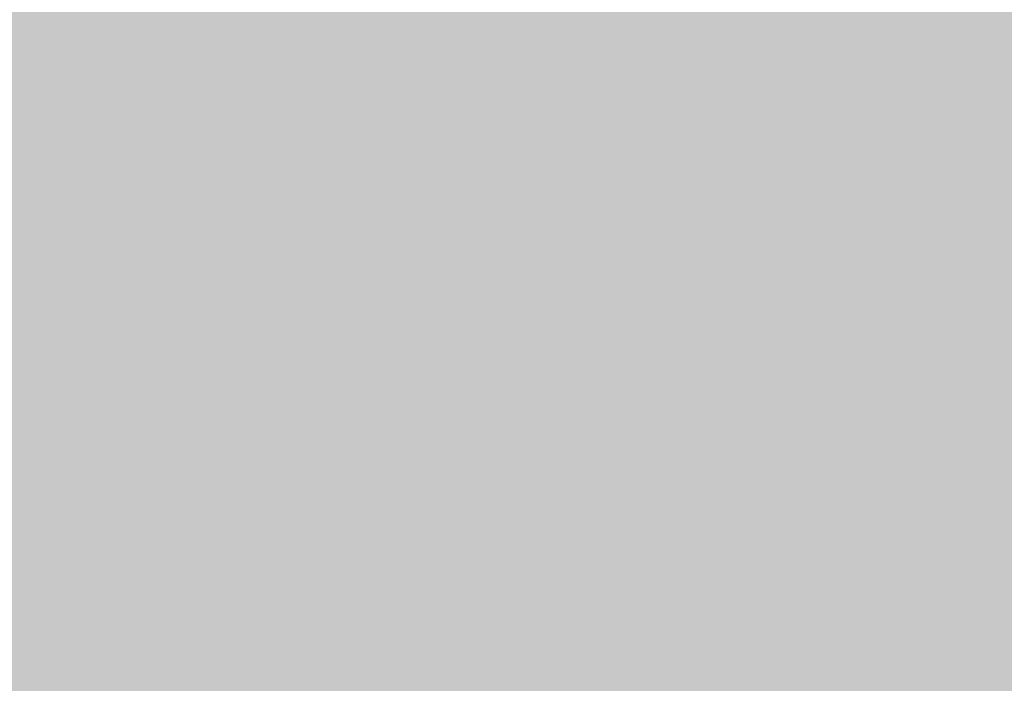
# Model space of a CAD drawing. Units: feet. Extents: x 3168 to 4724, y 827 to 1477.
# Tile 143 of 256: x 3301.1362 to 3301.138323, y 1099.01485 to 1099.016281. Entities that reach past the tile are written whole.
import ezdxf

# ---------------------------------------------------------------- set-up
doc = ezdxf.new("R2010")
doc.units = ezdxf.units.FT
doc.layers.add('A-ELEV', color=7, linetype='Continuous', lineweight=35)
doc.layers.add('A-ELEV-PATT', color=8, linetype='Continuous', lineweight=13)

msp = doc.modelspace()

# ---------------------------------------------------------------- hatches: boundary and pattern name
at = {"layer": 'A-ELEV-PATT'}
h = msp.add_hatch(color=256, dxfattribs=at)
h.dxf.hatch_style = 1
edge = h.paths.add_edge_path()
edge.add_ellipse((3552.9057615, 979.2201412), major_axis=(36.7449243, 0), ratio=0.4848484848, start_angle=0, end_angle=360)
edge = h.paths.add_edge_path()
edge.add_ellipse((3559.8916366, 929.2522824), major_axis=(36.7449243, 0), ratio=0.4848484848, start_angle=0, end_angle=360)
edge = h.paths.add_edge_path()
edge.add_line((3299.3168105, 1198.606081), (3479.9167135, 1198.606081))
edge.add_line((3479.9167135, 1198.606081), (3479.9167135, 1209.8685704))
edge.add_spline(control_points=[(3479.9167135, 1209.8685704), (3464.3011571, 1209.8685704), (3448.6856007, 1209.8685704), (3410.949139, 1209.8685704), (3388.8282339, 1209.8685704), (3355.6468761, 1209.8685704), (3344.5864235, 1209.8685704), (3327.9957446, 1209.8685704), (3322.4655183, 1209.8685704), (3314.1701788, 1209.8685704), (3311.4050657, 1209.8685704), (3307.257396, 1209.8685704), (3305.8748394, 1209.8685704), (3303.8010045, 1209.8685704), (3303.1097262, 1209.8685704), (3302.0728088, 1209.8685704), (3301.7271697, 1209.8685704), (3301.2087109, 1209.8685704), (3301.0358914, 1209.8685704), (3300.776662, 1209.8685704), (3300.6902522, 1209.8685704), (3300.5606376, 1209.8685704), (3300.5174327, 1209.8685704), (3300.4526253, 1209.8685704), (3300.4310229, 1209.8685704), (3300.3986192, 1209.8685704), (3300.387818, 1209.8685704), (3300.3662155, 1209.8685704), (3300.3456757, 1209.8685704), (3300.3455476, 1209.8685704), (3300.345505, 1209.8685704), (3300.3433041, 1209.8685704), (3300.341146, 1209.8685707), (3300.337909, 1209.8685714), (3300.33683, 1209.8685718), (3300.3339422, 1209.8685728), (3300.3321334, 1209.8685736), (3300.3255154, 1209.8685773), (3300.3207065, 1209.8685812), (3300.3109248, 1209.8685917), (3300.305952, 1209.8685984), (3300.2905113, 1209.8686233), (3300.2800452, 1209.8686461), (3300.2324255, 1209.868777), (3300.1952979, 1209.868954), (3299.9510684, 1209.8706077), (3299.7448244, 1209.8743259), (3299.4368271, 1209.8832566), (3299.3343894, 1209.8867924), (3299.181079, 1209.8929197), (3299.1300333, 1209.8950994), (3298.6522171, 1209.9168011), (3298.2294605, 1209.9457176), (3297.6016312, 1210.0023671), (3297.3934043, 1210.0234637), (3297.082652, 1210.058309), (3296.9793324, 1210.0704575), (3296.2929541, 1210.1548606), (3295.7181475, 1210.2433556), (3294.8687167, 1210.3988504), (3294.5876997, 1210.4544779), (3294.1693407, 1210.5433488), (3294.0304153, 1210.5738777), (3291.7071487, 1211.1012), (3289.6535901, 1211.8134353), (3285.7762586, 1213.5639876), (3283.9514101, 1214.6034778), (3280.512159, 1216.9800798), (3278.8972407, 1218.3175918), (3276.3799143, 1220.829489), (3275.4160415, 1221.9177379), (3274.0393421, 1223.7076996), (3273.5810428, 1224.3495346), (3273.1432283, 1225.0163162)], knot_values=[39.119033, 39.119033, 39.119033, 39.119033, 39.286353, 39.286353, 39.523379, 39.523379, 39.641892, 39.641892, 39.701148, 39.701148, 39.730777, 39.730777, 39.745591, 39.745591, 39.752998, 39.752998, 39.756701, 39.756701, 39.758553, 39.758553, 39.759479, 39.759479, 39.759942, 39.759942, 39.760173, 39.760173, 39.760289, 39.760289, 39.760405, 39.760405, 39.760463, 39.760463, 39.763389, 39.763389, 39.764851, 39.764851, 39.767304, 39.767304, 39.773825, 39.773825, 39.78057, 39.78057, 39.79477, 39.79477, 39.845194, 39.845194, 40.126715, 40.126715, 40.267476, 40.267476, 40.337856, 40.337856, 40.927023, 40.927023, 41.221606, 41.221606, 41.368898, 41.368898, 42.202622, 42.202622, 42.619485, 42.619485, 42.827916, 42.827916, 46.118323, 46.118323, 49.408731, 49.408731, 52.699139, 52.699139, 54.927489, 54.927489, 56.104228, 56.104228, 56.104228, 56.104228], weights=[1, 1, 1, 1, 1, 1, 1, 1, 1, 1, 1, 1, 1, 1, 1, 1, 1, 1, 1, 1, 1, 1, 1, 1, 1, 1, 1, 1, 1, 1, 1, 1, 1, 1, 1, 1, 1, 1, 1, 1, 1, 1, 1, 1, 1, 1, 1, 1, 1, 1, 1, 1, 1, 1, 1, 1, 1, 1, 1, 1, 1, 1, 1, 1, 1, 1, 1, 1, 1, 1, 1, 1, 1, 1], degree=3, periodic=0)
edge.add_line((3273.1432283, 1225.0163162), (3273.1432283, 1099.0163162))
edge.add_line((3273.1432283, 1099.0163162), (3299.3168105, 1099.0163162))
edge.add_line((3299.3168105, 1099.0163162), (3299.3168105, 1198.606081))
edge = h.paths.add_edge_path()
edge.add_line((3304.7584434, 1324.15806), (3479.9167135, 1324.15806))
edge.add_line((3479.9167135, 1324.15806), (3479.9167135, 1335.7146184))
edge.add_line((3479.9167135, 1335.7146184), (3269.1616284, 1335.7146184))
edge.add_spline(control_points=[(3269.1616284, 1335.7146184), (3264.0242315, 1335.7146184), (3258.364118, 1328.9581888), (3259.2643109, 1323.9002743)], knot_values=[0, 0, 0, 0, 15.412191, 15.412191, 15.412191, 15.412191], degree=3, periodic=0)
edge.add_line((3259.2643109, 1323.9002743), (3265.5168487, 1288.7691348))
edge.add_line((3265.5168487, 1288.7691348), (3275.2651026, 1261.5456259))
edge.add_line((3275.2651026, 1261.5456259), (3304.7584434, 1261.5456259))
edge.add_line((3304.7584434, 1261.5456259), (3304.7584434, 1324.15806))
h = msp.add_hatch(color=256, dxfattribs=at)
h.dxf.hatch_style = 1
h.paths.add_polyline_path([(3384.5252473, 1099.0163162), (3335.0291678, 1099.0163162), (3299.3168105, 1099.0163162), (3273.1432283, 1099.0163162), (3217.5653642, 1099.0163162), (3168.0692847, 827.1162598), (3335.0291678, 827.1162598)])

# ---------------------------------------------------------------- linework, layer by layer
at = {"layer": 'A-ELEV'}
msp.add_open_spline([(3808.5202001, 1099.0163162), (3808.5202001, 1141.413235), (3808.5202001, 1183.8101539), (3808.5202001, 1226.6353244), (3808.5202001, 1227.0635761), (3808.5202001, 1227.4918279), (3811.491871, 1248.9946729), (3814.463542, 1270.497518), (3817.4652299, 1292.2175635), (3817.4952467, 1292.434764), (3817.5252636, 1292.6519644), (3817.5728014, 1310.1067483), (3817.6203393, 1327.5615322), (3817.6678771, 1345.0163162), (3817.6678771, 1345.4579619), (3817.6678771, 1345.8996077), (3817.6678771, 1346.4560466), (3817.6678771, 1346.5708398), (3817.6678771, 1346.7528874), (3817.6678771, 1346.8201418), (3817.6678771, 1346.9348705), (3817.6678771, 1346.9823447), (3817.6678771, 1347.0385872), (3817.6678771, 1347.0473556), (3817.6678771, 1347.0736607), (3817.667877, 1347.0593025), (3817.6678766, 1347.0615455), (3817.6678764, 1347.0626669), (3817.6678754, 1347.0660311), (3817.6678743, 1347.0682738), (3817.6678701, 1347.0750012), (3817.667866, 1347.0794856), (3817.6678493, 1347.0929368), (3817.6678325, 1347.1019019), (3817.6677657, 1347.1287896), (3817.6676988, 1347.1467049), (3817.6674317, 1347.2004211), (3817.6671649, 1347.2361922), (3817.6661003, 1347.3433849), (3817.6650383, 1347.4146859), (3817.6608124, 1347.6280949), (3817.6566084, 1347.7697085), (3817.6399698, 1348.1924868), (3817.6235091, 1348.4715855), (3817.5590944, 1349.3000666), (3817.4961208, 1349.8405878), (3817.2554319, 1351.4241561), (3817.0263177, 1352.4287852), (3816.3068713, 1354.8889138), (3815.7437452, 1356.2687272), (3814.4639586, 1358.8192105), (3813.7464132, 1359.9909676), (3812.1958378, 1362.1723433), (3811.3622453, 1363.1821237), (3809.5888357, 1365.0690087), (3808.6488164, 1365.9461052), (3806.6542623, 1367.5796162), (3805.5997024, 1368.336154), (3803.3528906, 1369.7223272), (3802.1605354, 1370.352386), (3799.6008131, 1371.4535864), (3798.2326878, 1371.9254812), (3795.2800838, 1372.6346239), (3793.6931479, 1372.8720685), (3791.8694413, 1372.9264797), (3791.7408615, 1372.9292203), (3791.3533713, 1372.9341014), (3791.0927074, 1372.9329013), (3790.3041163, 1372.9150676), (3789.7695426, 1372.8841946), (3789.20919, 1372.8302363), (3789.1906217, 1372.8284241), (3789.1348916, 1372.8229123), (3789.097705, 1372.8191375), (3789.0484446, 1372.8140077), (3789.0364001, 1372.8127432), (3789.0002562, 1372.808918), (3788.9761468, 1372.8063255), (3788.9494049, 1372.8034042), (3788.9467858, 1372.8031177), (3788.9425667, 1372.8026552), (3788.9409669, 1372.8024797), (3788.9385718, 1372.8022166), (3788.9377765, 1372.8021292), (3788.9353908, 1372.8018669), (3788.8675349, 1372.7944024), (3788.7568665, 1372.7822285), (3788.7015323, 1372.7761415), (3788.5355297, 1372.7578805), (3788.4248612, 1372.7457065), (3788.092856, 1372.7091846), (3787.8715192, 1372.6848366), (3787.2075086, 1372.6117927), (3786.764835, 1372.5630968), (3785.436814, 1372.417009), (3784.5514666, 1372.3196171), (3781.8954246, 1372.0274416), (3780.1247299, 1371.8326579), (3774.8126458, 1371.2483067), (3771.2712564, 1370.8587393), (3760.6470883, 1369.6900371), (3753.5643095, 1368.9109022), (3732.3159732, 1366.5734977), (3718.1504157, 1365.015228), (3694.0067577, 1362.3593262), (3684.0286573, 1361.2616941), (3674.0505568, 1360.1640619), (3664.6006617, 1360.1640619), (3655.1507666, 1360.1640619), (3626.8010812, 1360.1640619), (3607.9012909, 1360.1640619), (3551.2019201, 1360.1640619), (3513.4023395, 1360.1640619), (3467.7251817, 1360.1640619), (3459.8476045, 1360.1640619), (3436.2148727, 1360.1640619), (3420.4597182, 1360.1640619), (3373.1942547, 1360.1640619), (3341.6839457, 1360.1640619), (3302.8481616, 1360.1640619), (3295.5226865, 1360.1640619), (3286.0382916, 1360.1640619), (3283.8793719, 1360.1640619), (3277.4026128, 1360.1640619), (3273.0847733, 1360.1640619), (3267.7328511, 1360.1640619), (3266.6987684, 1360.1640619), (3263.5965201, 1360.1640619), (3261.5283546, 1360.1640619), (3259.2369429, 1360.1640619), (3259.0136967, 1360.1640619), (3258.3439582, 1360.1640619), (3257.8974658, 1360.1640619), (3257.4309979, 1360.1640619), (3257.4110224, 1360.1640619), (3257.3705735, 1360.1640619), (3257.3754695, 1360.1640619), (3257.3745975, 1360.1640619), (3257.3739371, 1360.1640618), (3257.3719559, 1360.1640616), (3257.3706351, 1360.1640613), (3257.366673, 1360.16406), (3257.3640318, 1360.1640586), (3257.3561088, 1360.1640529), (3257.3508277, 1360.1640469), (3257.3349869, 1360.1640226), (3257.3244299, 1360.163998), (3257.2927692, 1360.1638987), (3257.2716761, 1360.1637987), (3257.208439, 1360.1633975), (3257.1663373, 1360.1629953), (3257.0402058, 1360.1613882), (3256.9563493, 1360.1597827), (3256.705504, 1360.1533932), (3256.53924, 1360.1470361), (3256.0435702, 1360.1219156), (3255.717296, 1360.0971018), (3254.7524458, 1360.0004808), (3254.1279679, 1359.906513), (3252.1800666, 1359.5253322), (3250.9415739, 1359.1439911), (3248.6701751, 1358.2432905), (3247.6357388, 1357.7238339), (3245.7326321, 1356.6034712), (3244.8633884, 1356.0020595), (3243.2531076, 1354.7428655), (3242.511972, 1354.0847309), (3240.7510518, 1352.3447812), (3239.8009609, 1351.229574), (3238.0877694, 1348.8724402), (3237.3246853, 1347.6303552), (3235.9825098, 1344.9716321), (3235.4022051, 1343.554907), (3234.5910812, 1340.8154577), (3234.3108819, 1339.5435498), (3233.9764902, 1336.8025605), (3233.9221126, 1335.3308771), (3234.1489156, 1332.5912693), (3234.3495287, 1331.3672011), (3234.7198926, 1329.9993668), (3234.7524228, 1329.8833616), (3234.853619, 1329.5347966), (3234.9258923, 1329.301685), (3235.0248359, 1329.0025524), (3235.0469235, 1328.936928), (3235.0776388, 1328.8472393), (3235.0859239, 1328.8231979), (3235.1109389, 1328.7510642), (3235.1278282, 1328.7029624), (3235.1479919, 1328.6462418), (3235.1510592, 1328.6376324), (3235.1560959, 1328.6235265), (3235.1580611, 1328.6180301), (3235.1602094, 1328.6120302), (3235.1656119, 1328.596943), (3235.1800989, 1328.556486), (3235.190263, 1328.5281009), (3235.2207556, 1328.4429457), (3235.241084, 1328.3861755), (3235.3020692, 1328.215865), (3235.3427259, 1328.1023247), (3235.4646962, 1327.7617038), (3235.5460097, 1327.5346232), (3235.7899503, 1326.8533813), (3235.9525774, 1326.39922), (3236.4404586, 1325.0367362), (3236.7657127, 1324.1284137), (3237.7414751, 1321.4034462), (3238.3919833, 1319.5868011), (3240.3435081, 1314.136866), (3241.6445245, 1310.503576), (3245.547574, 1299.6037058), (3248.149607, 1292.3371257), (3255.955706, 1270.5373853), (3261.1597719, 1256.004225), (3267.3876177, 1238.6120011), (3268.4113975, 1235.7529374), (3269.5103781, 1232.6838639), (3269.5855789, 1232.473854), (3269.7066118, 1232.1358507), (3269.752444, 1232.0078573), (3269.8273289, 1231.7987296), (3269.8563817, 1231.7175953), (3269.9063247, 1231.5781217), (3269.927215, 1231.5197823), (3269.9724682, 1231.3934057), (3269.9968311, 1231.3253685), (3270.0265026, 1231.2425062), (3270.0318112, 1231.2276812), (3270.0402823, 1231.2040243), (3270.0392242, 1231.2069792), (3270.0393595, 1231.2066014), (3270.0394271, 1231.2064125), (3270.0396301, 1231.2058458), (3270.0397654, 1231.205468), (3270.0401713, 1231.2043346), (3270.040442, 1231.2035791), (3270.041254, 1231.2013125), (3270.0417955, 1231.1998016), (3270.0434203, 1231.195269), (3270.044504, 1231.1922477), (3270.0477563, 1231.1831849), (3270.0499263, 1231.1771446), (3270.0564418, 1231.1590283), (3270.0607927, 1231.146957), (3270.0738674, 1231.1107614), (3270.0826128, 1231.0866558), (3270.1089357, 1231.0144129), (3270.1265997, 1230.9663498), (3270.1799341, 1230.8224568), (3270.2159467, 1230.7269233), (3270.3253234, 1230.4415078), (3270.4000257, 1230.2528107), (3270.6292491, 1229.6914436), (3270.7888829, 1229.3235005), (3271.2864875, 1228.2383194), (3271.6430996, 1227.5397546), (3272.7758592, 1225.515277), (3273.6141694, 1224.2605021), (3275.4160415, 1221.9177379), (3276.3799143, 1220.829489), (3278.8972407, 1218.3175918), (3280.512159, 1216.9800798), (3283.9514101, 1214.6034778), (3285.7762586, 1213.5639876), (3289.6535901, 1211.8134353), (3291.7071487, 1211.1012), (3294.0304153, 1210.5738777), (3294.1693407, 1210.5433488), (3294.5876997, 1210.4544779), (3294.8687167, 1210.3988504), (3295.7181475, 1210.2433556), (3296.2929541, 1210.1548606), (3296.9793324, 1210.0704575), (3297.082652, 1210.058309), (3297.3934043, 1210.0234637), (3297.6016312, 1210.0023671), (3298.2294605, 1209.9457176), (3298.6522171, 1209.9168011), (3299.1300333, 1209.8950994), (3299.181079, 1209.8929197), (3299.3343894, 1209.8867924), (3299.4368271, 1209.8832566), (3299.7448244, 1209.8743259), (3299.9510684, 1209.8706077), (3300.1952979, 1209.868954), (3300.2324255, 1209.868777), (3300.2800452, 1209.8686461), (3300.2905113, 1209.8686233), (3300.305952, 1209.8685984), (3300.3109248, 1209.8685917), (3300.3207065, 1209.8685812), (3300.3255154, 1209.8685773), (3300.3321334, 1209.8685736), (3300.3339422, 1209.8685728), (3300.33683, 1209.8685718), (3300.337909, 1209.8685714), (3300.341146, 1209.8685707), (3300.3433041, 1209.8685704), (3300.345505, 1209.8685704), (3300.3455476, 1209.8685704), (3300.3456757, 1209.8685704), (3300.3662155, 1209.8685704), (3300.387818, 1209.8685704), (3300.3986192, 1209.8685704), (3300.4310229, 1209.8685704), (3300.4526253, 1209.8685704), (3300.5174327, 1209.8685704), (3300.5606376, 1209.8685704), (3300.6902522, 1209.8685704), (3300.776662, 1209.8685704), (3301.0358914, 1209.8685704), (3301.2087109, 1209.8685704), (3301.7271697, 1209.8685704), (3302.0728088, 1209.8685704), (3303.1097262, 1209.8685704), (3303.8010045, 1209.8685704), (3305.8748394, 1209.8685704), (3307.257396, 1209.8685704), (3311.4050657, 1209.8685704), (3314.1701788, 1209.8685704), (3322.4655183, 1209.8685704), (3327.9957446, 1209.8685704), (3344.5864235, 1209.8685704), (3355.6468761, 1209.8685704), (3388.8282339, 1209.8685704), (3410.949139, 1209.8685704), (3477.3118546, 1209.8685704), (3521.553665, 1209.8685704), (3566.8361836, 1209.8685704), (3567.8768919, 1209.8685704), (3570.9990167, 1209.8685704), (3573.0804332, 1209.8685704), (3575.7813964, 1209.8685704), (3576.4009432, 1209.8685704), (3577.2958211, 1209.8685704), (3577.5711523, 1209.8685704), (3578.3971458, 1209.8685704), (3578.9478081, 1209.8685704), (3579.7564907, 1209.8685704), (3580.0145108, 1209.8685704), (3580.3427367, 1209.8685704), (3580.3268649, 1209.8685704), (3580.3271702, 1209.8685704), (3580.3273229, 1209.8685704), (3580.3277809, 1209.8685704), (3580.3280863, 1209.8685704), (3580.3290024, 1209.8685703), (3580.3296132, 1209.8685702), (3580.3314455, 1209.8685699), (3580.332667, 1209.8685697), (3580.336332, 1209.8685685), (3580.3387755, 1209.8685674), (3580.3461066, 1209.8685629), (3580.350995, 1209.8685584), (3580.3656627, 1209.8685402), (3580.3754446, 1209.868522), (3580.4048012, 1209.8684493), (3580.4243863, 1209.8683764), (3580.4831833, 1209.8680848), (3580.5224371, 1209.8677929), (3580.6403612, 1209.8666242), (3580.7191947, 1209.8654543), (3580.9563152, 1209.8607663), (3581.1152222, 1209.85607), (3581.5941635, 1209.8372298), (3581.9164188, 1209.8183314), (3582.8899466, 1209.7424284), (3583.547986, 1209.6661692), (3585.5318268, 1209.3606172), (3586.8672159, 1209.0538859), (3589.4715454, 1208.2524717), (3590.7402412, 1207.7578521), (3591.9954511, 1207.1588024), (3592.057809, 1207.1287398), (3592.2442418, 1207.0379536), (3592.3676757, 1206.9766317), (3592.73528, 1206.7903591), (3592.9767518, 1206.663101), (3593.2445387, 1206.5164414), (3593.2747313, 1206.4998248), (3593.3651153, 1206.4498388), (3593.4251129, 1206.4163333), (3593.6043138, 1206.3152851), (3593.7227254, 1206.2472105), (3593.8572122, 1206.1683978), (3593.8743621, 1206.1583193), (3593.925741, 1206.1280407), (3593.9598989, 1206.1077976), (3594.0620855, 1206.0468991), (3594.1298272, 1206.0060745), (3594.2084359, 1205.9581709), (3594.2196829, 1205.9513043), (3594.253391, 1205.9306863), (3594.2758193, 1205.9169166), (3594.3429716, 1205.8755358), (3594.3875633, 1205.8478526), (3594.4336161, 1205.8190499), (3594.4352559, 1205.818024), (3594.4401746, 1205.8149461), (3594.4434527, 1205.8128936), (3594.4471229, 1205.8105944), (3594.4475159, 1205.8103482), (3594.4486949, 1205.8096095), (3594.4494808, 1205.8091171), (3594.4503663, 1205.8085621), (3594.4504658, 1205.8084998), (3594.4506003, 1205.8084155), (3594.4673993, 1205.7978872), (3594.4932689, 1205.7816741), (3594.5062037, 1205.7735675), (3594.5450081, 1205.7492479), (3594.5708778, 1205.7330348), (3594.6484866, 1205.6843956), (3594.7002258, 1205.6519694), (3594.8554436, 1205.5546909), (3594.958922, 1205.4898386), (3595.2693574, 1205.2952816), (3595.4763144, 1205.1655769), (3596.0971852, 1204.7764629), (3596.5110991, 1204.5170536), (3597.7528407, 1203.7388256), (3598.5806685, 1203.220007), (3601.0641518, 1201.663551), (3602.7198073, 1200.6259137), (3607.686774, 1197.5130018), (3610.998085, 1195.4377272), (3620.9320182, 1189.2119034), (3627.5546404, 1185.0613542), (3647.4225068, 1172.6097066), (3660.6677511, 1164.3086082), (3700.403484, 1139.405313), (3726.8939725, 1122.8031161), (3757.2057154, 1103.8060516), (3761.0269697, 1101.4111839), (3764.848224, 1099.0163162), (3745.3282713, 1099.0163162), (3725.8083186, 1099.0163162), (3706.288366, 1099.0163162), (3706.288366, 1108.4532371), (3706.288366, 1117.890158), (3706.288366, 1127.3270789), (3710.7507544, 1127.3270789), (3715.2131428, 1127.3270789), (3719.6755312, 1127.3270789)], degree=3, knots=[0, 0, 0, 0, 0.982037, 0.982037, 0.991957, 0.991957, 0.991957, 1.966522, 1.966522, 1.976367, 1.976367, 1.976367, 2.976367, 2.976367, 2.976367, 3.00169, 3.00169, 3.008272, 3.008272, 3.012129, 3.012129, 3.014851, 3.014851, 3.015353, 3.015353, 3.016359, 3.016359, 3.017365, 3.017365, 3.019376, 3.019376, 3.023398, 3.023398, 3.031442, 3.031442, 3.047531, 3.047531, 3.079708, 3.079708, 3.144063, 3.144063, 3.272772, 3.272772, 3.53019, 3.53019, 4.045026, 4.045026, 5.074698, 5.074698, 6.700878, 6.700878, 8.327058, 8.327058, 9.953238, 9.953238, 11.579418, 11.579418, 13.205598, 13.205598, 14.831778, 14.831778, 16.457958, 16.457958, 18.084138, 18.084138, 18.206872, 18.206872, 18.45234, 18.45234, 18.943275, 18.943275, 18.960093, 18.960093, 18.993729, 18.993729, 19.00461, 19.00461, 19.026374, 19.026374, 19.028737, 19.028737, 19.03018, 19.03018, 19.030897, 19.030897, 19.032332, 19.032332, 19.033766, 19.033766, 19.036636, 19.036636, 19.042374, 19.042374, 19.053851, 19.053851, 19.076805, 19.076805, 19.122714, 19.122714, 19.21453, 19.21453, 19.398163, 19.398163, 19.765429, 19.765429, 20.024128, 20.024128, 20.024128, 20.092031, 20.092031, 20.227836, 20.227836, 20.499446, 20.499446, 20.556051, 20.556051, 20.66926, 20.66926, 20.895678, 20.895678, 20.948316, 20.948316, 20.963829, 20.963829, 20.994855, 20.994855, 21.002285, 21.002285, 21.017146, 21.017146, 21.01875, 21.01875, 21.021959, 21.021959, 21.022102, 21.022102, 21.022249, 21.022249, 21.022708, 21.022708, 21.023627, 21.023627, 21.025464, 21.025464, 21.029138, 21.029138, 21.036486, 21.036486, 21.051183, 21.051183, 21.080575, 21.080575, 21.139361, 21.139361, 21.256932, 21.256932, 21.492073, 21.492073, 21.962356, 21.962356, 23.01002, 23.01002, 24.057684, 24.057684, 25.105348, 25.105348, 26.153011, 26.153011, 27.776787, 27.776787, 29.400562, 29.400562, 31.024337, 31.024337, 32.278801, 32.278801, 33.533265, 33.533265, 34.467568, 34.467568, 34.553971, 34.553971, 34.726776, 34.726776, 34.775309, 34.775309, 34.793079, 34.793079, 34.82862, 34.82862, 34.834979, 34.834979, 34.839039, 34.839039, 34.839411, 34.839411, 34.840285, 34.840285, 34.842034, 34.842034, 34.845531, 34.845531, 34.852525, 34.852525, 34.866512, 34.866512, 34.894488, 34.894488, 34.950439, 34.950439, 35.062342, 35.062342, 35.286147, 35.286147, 35.733758, 35.733758, 35.821815, 35.821815, 35.828283, 35.828283, 35.832225, 35.832225, 35.834724, 35.834724, 35.836521, 35.836521, 35.838617, 35.838617, 35.839073, 35.839073, 35.839345, 35.839345, 35.839617, 35.839617, 35.840161, 35.840161, 35.841249, 35.841249, 35.843425, 35.843425, 35.847778, 35.847778, 35.856482, 35.856482, 35.873891, 35.873891, 35.908709, 35.908709, 35.978345, 35.978345, 36.117617, 36.117617, 36.396161, 36.396161, 36.953248, 36.953248, 38.067423, 38.067423, 40.295772, 40.295772, 42.524122, 42.524122, 45.81453, 45.81453, 49.104937, 49.104937, 52.395345, 52.395345, 52.603776, 52.603776, 53.020639, 53.020639, 53.854363, 53.854363, 54.001655, 54.001655, 54.296238, 54.296238, 54.885405, 54.885405, 54.955785, 54.955785, 55.096546, 55.096546, 55.378067, 55.378067, 55.42849, 55.42849, 55.442691, 55.442691, 55.449436, 55.449436, 55.455957, 55.455957, 55.458409, 55.458409, 55.459872, 55.459872, 55.462798, 55.462798, 55.462856, 55.462856, 55.462972, 55.462972, 55.463088, 55.463088, 55.463319, 55.463319, 55.463782, 55.463782, 55.464708, 55.464708, 55.46656, 55.46656, 55.470263, 55.470263, 55.47767, 55.47767, 55.492484, 55.492484, 55.522112, 55.522112, 55.581369, 55.581369, 55.699882, 55.699882, 55.936907, 55.936907, 56.410959, 56.410959, 56.42211, 56.42211, 56.444413, 56.444413, 56.451051, 56.451051, 56.454001, 56.454001, 56.459901, 56.459901, 56.462666, 56.462666, 56.463418, 56.463418, 56.464171, 56.464171, 56.465675, 56.465675, 56.468684, 56.468684, 56.474702, 56.474702, 56.486738, 56.486738, 56.51081, 56.51081, 56.558955, 56.558955, 56.655243, 56.655243, 56.847821, 56.847821, 57.232975, 57.232975, 58.003284, 58.003284, 59.543901, 59.543901, 62.625137, 62.625137, 68.787607, 68.787607, 74.950078, 74.950078, 75.27336, 75.27336, 75.919923, 75.919923, 77.213051, 77.213051, 77.377769, 77.377769, 77.707206, 77.707206, 78.366079, 78.366079, 78.462532, 78.462532, 78.655436, 78.655436, 79.041245, 79.041245, 79.105735, 79.105735, 79.234714, 79.234714, 79.492672, 79.492672, 79.502197, 79.502197, 79.521249, 79.521249, 79.523534, 79.523534, 79.528103, 79.528103, 79.528682, 79.528682, 79.528885, 79.528885, 79.529089, 79.529089, 79.529495, 79.529495, 79.530308, 79.530308, 79.531935, 79.531935, 79.535187, 79.535187, 79.541693, 79.541693, 79.554704, 79.554704, 79.580725, 79.580725, 79.632769, 79.632769, 79.736856, 79.736856, 79.94503, 79.94503, 80.361377, 80.361377, 80.421435, 80.421435, 80.421435, 81.421435, 81.421435, 81.421435, 82.421435, 82.421435, 82.421435, 83.421435, 83.421435, 83.421435, 83.421435], dxfattribs=at)

doc.saveas('drawing.dxf')
